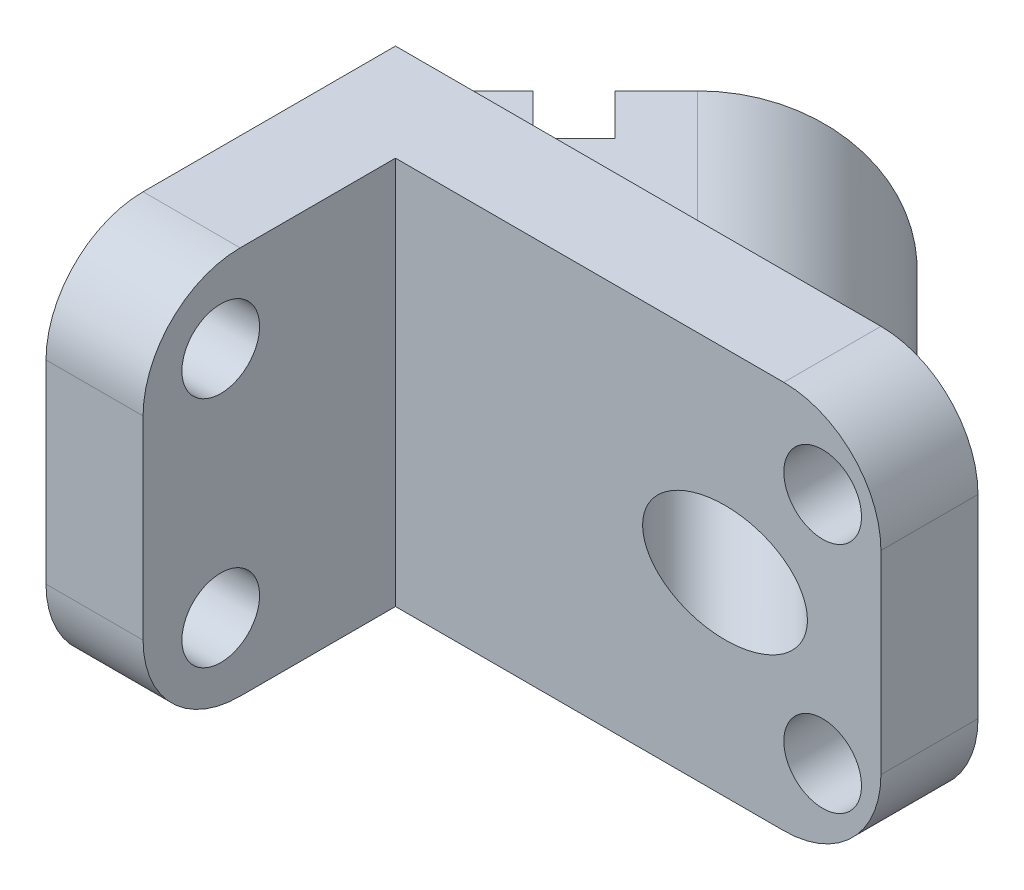
ISO-10303-21;
HEADER;
FILE_DESCRIPTION(('STEP AP214'),'2;1');
FILE_NAME('part.step','',(''),(''),'','','');
FILE_SCHEMA(('AUTOMOTIVE_DESIGN { 1 0 10303 214 1 1 1 1 }'));
ENDSEC;
DATA;
#1=APPLICATION_CONTEXT('core data for automotive mechanical design processes');
#2=APPLICATION_PROTOCOL_DEFINITION('international standard','automotive_design',2000,#1);
#3=PRODUCT_CONTEXT('',#1,'mechanical');
#4=PRODUCT('Part','Part','',(#3));
#5=PRODUCT_RELATED_PRODUCT_CATEGORY('part','',(#4));
#6=PRODUCT_DEFINITION_FORMATION('','',#4);
#7=PRODUCT_DEFINITION_CONTEXT('part definition',#1,'design');
#8=PRODUCT_DEFINITION('design','',#6,#7);
#9=PRODUCT_DEFINITION_SHAPE('','',#8);
#10=(LENGTH_UNIT() NAMED_UNIT(*) SI_UNIT(.MILLI.,.METRE.));
#11=(NAMED_UNIT(*) PLANE_ANGLE_UNIT() SI_UNIT($,.RADIAN.));
#12=(NAMED_UNIT(*) SI_UNIT($,.STERADIAN.) SOLID_ANGLE_UNIT());
#13=UNCERTAINTY_MEASURE_WITH_UNIT(LENGTH_MEASURE(1.E-05),#10,'distance_accuracy_value','');
#14=(GEOMETRIC_REPRESENTATION_CONTEXT(3) GLOBAL_UNCERTAINTY_ASSIGNED_CONTEXT((#13)) GLOBAL_UNIT_ASSIGNED_CONTEXT((#10,
#11,#12)) REPRESENTATION_CONTEXT('',''));
#15=CARTESIAN_POINT('',(0.,0.,0.));
#16=DIRECTION('',(0.,0.,1.));
#17=DIRECTION('',(1.,0.,0.));
#18=AXIS2_PLACEMENT_3D('',#15,#16,#17);
#19=CARTESIAN_POINT('',(-36.1091270347396,0.,-38.8908729652601));
#20=DIRECTION('',(0.707106781186544,0.,0.707106781186551));
#21=DIRECTION('',(0.707106781186551,0.,-0.707106781186544));
#22=AXIS2_PLACEMENT_3D('',#19,#20,#21);
#23=PLANE('',#22);
#24=DIRECTION('',(-0.707106781186551,0.,0.707106781186544));
#25=VECTOR('',#24,1.);
#26=CARTESIAN_POINT('',(-74.9999999999999,40.,-1.38777878078145E-13));
#27=LINE('',#26,#25);
#28=CARTESIAN_POINT('',(-57.3223304703362,40.,-17.6776695296636));
#29=VERTEX_POINT('',#28);
#30=CARTESIAN_POINT('',(-75.,40.,0.));
#31=VERTEX_POINT('',#30);
#32=EDGE_CURVE('E201',#29,#31,#27,.T.);
#33=ORIENTED_EDGE('',*,*,#32,.F.);
#34=DIRECTION('',(0.,1.,0.));
#35=VECTOR('',#34,1.);
#36=CARTESIAN_POINT('',(-57.3223304703362,-50.001,-17.6776695296636));
#37=LINE('',#36,#35);
#38=CARTESIAN_POINT('',(-57.3223304703362,-40.,-17.6776695296636));
#39=VERTEX_POINT('',#38);
#40=EDGE_CURVE('E200',#39,#29,#37,.T.);
#41=ORIENTED_EDGE('',*,*,#40,.F.);
#42=DIRECTION('',(0.707106781186551,0.,-0.707106781186544));
#43=VECTOR('',#42,1.);
#44=CARTESIAN_POINT('',(-74.9999999999999,-40.,-1.38777878078145E-13));
#45=LINE('',#44,#43);
#46=CARTESIAN_POINT('',(-74.9999999999999,-40.,-1.38777878078145E-13));
#47=VERTEX_POINT('',#46);
#48=EDGE_CURVE('E202',#47,#39,#45,.T.);
#49=ORIENTED_EDGE('',*,*,#48,.F.);
#50=DIRECTION('',(0.,-1.,0.));
#51=VECTOR('',#50,1.);
#52=CARTESIAN_POINT('',(-74.9999999999999,40.,-1.38777878078145E-13));
#53=LINE('',#52,#51);
#54=EDGE_CURVE('E207',#31,#47,#53,.T.);
#55=ORIENTED_EDGE('',*,*,#54,.F.);
#56=EDGE_LOOP('',(#33,#41,#49,#55));
#57=FACE_BOUND('',#56,.T.);
#58=ADVANCED_FACE('F39',(#57),#23,.F.);
#59=CARTESIAN_POINT('',(0.,0.,25.));
#60=DIRECTION('',(0.,0.,-1.));
#61=DIRECTION('',(-1.,0.,0.));
#62=AXIS2_PLACEMENT_3D('',#59,#60,#61);
#63=PLANE('',#62);
#64=CARTESIAN_POINT('',(60.,30.,25.));
#65=DIRECTION('',(0.,0.,-1.));
#66=DIRECTION('',(-1.,0.,0.));
#67=AXIS2_PLACEMENT_3D('',#64,#65,#66);
#68=CIRCLE('',#67,10.);
#69=CARTESIAN_POINT('',(50.,30.,25.));
#70=VERTEX_POINT('',#69);
#71=EDGE_CURVE('E597',#70,#70,#68,.F.);
#72=ORIENTED_EDGE('',*,*,#71,.F.);
#73=EDGE_LOOP('',(#72));
#74=FACE_BOUND('',#73,.T.);
#75=CARTESIAN_POINT('',(60.,-30.,25.));
#76=DIRECTION('',(0.,0.,-1.));
#77=DIRECTION('',(-1.,0.,0.));
#78=AXIS2_PLACEMENT_3D('',#75,#76,#77);
#79=CIRCLE('',#78,10.);
#80=CARTESIAN_POINT('',(50.,-30.,25.));
#81=VERTEX_POINT('',#80);
#82=EDGE_CURVE('E585',#81,#81,#79,.F.);
#83=ORIENTED_EDGE('',*,*,#82,.F.);
#84=EDGE_LOOP('',(#83));
#85=FACE_BOUND('',#84,.T.);
#86=CARTESIAN_POINT('',(34.852813742385,0.,25.));
#87=DIRECTION('',(0.,0.,-1.));
#88=DIRECTION('',(-1.,0.,0.));
#89=AXIS2_PLACEMENT_3D('',#86,#87,#88);
#90=ELLIPSE('',#89,21.2132034355963,15.);
#91=CARTESIAN_POINT('',(13.6396103067887,0.,25.));
#92=VERTEX_POINT('',#91);
#93=EDGE_CURVE('E182',#92,#92,#90,.F.);
#94=ORIENTED_EDGE('',*,*,#93,.F.);
#95=EDGE_LOOP('',(#94));
#96=FACE_BOUND('',#95,.T.);
#97=DIRECTION('',(0.,1.,0.));
#98=VECTOR('',#97,1.);
#99=CARTESIAN_POINT('',(75.,-50.,25.));
#100=LINE('',#99,#98);
#101=CARTESIAN_POINT('',(75.,-25.,25.));
#102=VERTEX_POINT('',#101);
#103=CARTESIAN_POINT('',(75.,25.,25.));
#104=VERTEX_POINT('',#103);
#105=EDGE_CURVE('E237',#102,#104,#100,.T.);
#106=ORIENTED_EDGE('',*,*,#105,.T.);
#107=CARTESIAN_POINT('',(50.,25.,25.));
#108=DIRECTION('',(0.,0.,-1.));
#109=DIRECTION('',(-1.,0.,0.));
#110=AXIS2_PLACEMENT_3D('',#107,#108,#109);
#111=CIRCLE('',#110,25.);
#112=CARTESIAN_POINT('',(50.,50.,25.));
#113=VERTEX_POINT('',#112);
#114=EDGE_CURVE('E11',#104,#113,#111,.F.);
#115=ORIENTED_EDGE('',*,*,#114,.T.);
#116=DIRECTION('',(-1.,0.,0.));
#117=VECTOR('',#116,1.);
#118=CARTESIAN_POINT('',(-75.,50.,25.));
#119=LINE('',#118,#117);
#120=CARTESIAN_POINT('',(-50.,50.,25.));
#121=VERTEX_POINT('',#120);
#122=EDGE_CURVE('E241',#113,#121,#119,.T.);
#123=ORIENTED_EDGE('',*,*,#122,.T.);
#124=DIRECTION('',(0.,1.,0.));
#125=VECTOR('',#124,1.);
#126=CARTESIAN_POINT('',(-50.,50.,25.));
#127=LINE('',#126,#125);
#128=CARTESIAN_POINT('',(-50.,-50.,25.));
#129=VERTEX_POINT('',#128);
#130=EDGE_CURVE('E206',#129,#121,#127,.T.);
#131=ORIENTED_EDGE('',*,*,#130,.F.);
#132=DIRECTION('',(1.,0.,0.));
#133=VECTOR('',#132,1.);
#134=CARTESIAN_POINT('',(-75.,-50.,25.));
#135=LINE('',#134,#133);
#136=CARTESIAN_POINT('',(50.,-50.,25.));
#137=VERTEX_POINT('',#136);
#138=EDGE_CURVE('E242',#129,#137,#135,.T.);
#139=ORIENTED_EDGE('',*,*,#138,.T.);
#140=CARTESIAN_POINT('',(50.,-25.,25.));
#141=DIRECTION('',(0.,0.,-1.));
#142=DIRECTION('',(-1.,0.,0.));
#143=AXIS2_PLACEMENT_3D('',#140,#141,#142);
#144=CIRCLE('',#143,25.);
#145=EDGE_CURVE('E290',#137,#102,#144,.F.);
#146=ORIENTED_EDGE('',*,*,#145,.T.);
#147=EDGE_LOOP('',(#106,#115,#123,#131,#139,#146));
#148=FACE_BOUND('',#147,.T.);
#149=ADVANCED_FACE('F337',(#74,#85,#96,#148),#63,.F.);
#150=CARTESIAN_POINT('',(75.,-50.,25.));
#151=DIRECTION('',(-1.,0.,0.));
#152=DIRECTION('',(0.,0.,1.));
#153=AXIS2_PLACEMENT_3D('',#150,#151,#152);
#154=PLANE('',#153);
#155=DIRECTION('',(0.,1.,0.));
#156=VECTOR('',#155,1.);
#157=CARTESIAN_POINT('',(75.,-50.,0.));
#158=LINE('',#157,#156);
#159=CARTESIAN_POINT('',(75.,-25.,0.));
#160=VERTEX_POINT('',#159);
#161=CARTESIAN_POINT('',(75.,25.,0.));
#162=VERTEX_POINT('',#161);
#163=EDGE_CURVE('E238',#160,#162,#158,.T.);
#164=ORIENTED_EDGE('',*,*,#163,.T.);
#165=DIRECTION('',(0.,0.,-1.));
#166=VECTOR('',#165,1.);
#167=CARTESIAN_POINT('',(75.,25.,25.));
#168=LINE('',#167,#166);
#169=EDGE_CURVE('E50',#162,#104,#168,.F.);
#170=ORIENTED_EDGE('',*,*,#169,.T.);
#171=ORIENTED_EDGE('',*,*,#105,.F.);
#172=DIRECTION('',(0.,0.,-1.));
#173=VECTOR('',#172,1.);
#174=CARTESIAN_POINT('',(75.,-25.,25.));
#175=LINE('',#174,#173);
#176=EDGE_CURVE('E277',#102,#160,#175,.T.);
#177=ORIENTED_EDGE('',*,*,#176,.T.);
#178=EDGE_LOOP('',(#164,#170,#171,#177));
#179=FACE_BOUND('',#178,.T.);
#180=ADVANCED_FACE('F345',(#179),#154,.F.);
#181=CARTESIAN_POINT('',(-75.,50.,25.));
#182=DIRECTION('',(0.,-1.,0.));
#183=DIRECTION('',(0.,0.,-1.));
#184=AXIS2_PLACEMENT_3D('',#181,#182,#183);
#185=PLANE('',#184);
#186=ORIENTED_EDGE('',*,*,#122,.F.);
#187=DIRECTION('',(0.,0.,-1.));
#188=VECTOR('',#187,1.);
#189=CARTESIAN_POINT('',(50.,50.,25.));
#190=LINE('',#189,#188);
#191=CARTESIAN_POINT('',(50.,50.,0.));
#192=VERTEX_POINT('',#191);
#193=EDGE_CURVE('E287',#113,#192,#190,.T.);
#194=ORIENTED_EDGE('',*,*,#193,.T.);
#195=DIRECTION('',(-1.,0.,0.));
#196=VECTOR('',#195,1.);
#197=CARTESIAN_POINT('',(-75.,50.,0.));
#198=LINE('',#197,#196);
#199=CARTESIAN_POINT('',(-75.,50.,0.));
#200=VERTEX_POINT('',#199);
#201=EDGE_CURVE('E248',#192,#200,#198,.T.);
#202=ORIENTED_EDGE('',*,*,#201,.T.);
#203=DIRECTION('',(0.,0.,-1.));
#204=VECTOR('',#203,1.);
#205=CARTESIAN_POINT('',(-75.,50.,25.));
#206=LINE('',#205,#204);
#207=CARTESIAN_POINT('',(-75.,50.,65.));
#208=VERTEX_POINT('',#207);
#209=EDGE_CURVE('E260',#208,#200,#206,.T.);
#210=ORIENTED_EDGE('',*,*,#209,.F.);
#211=DIRECTION('',(-1.,0.,0.));
#212=VECTOR('',#211,1.);
#213=CARTESIAN_POINT('',(-50.,50.,65.));
#214=LINE('',#213,#212);
#215=CARTESIAN_POINT('',(-50.,50.,65.));
#216=VERTEX_POINT('',#215);
#217=EDGE_CURVE('E268',#208,#216,#214,.F.);
#218=ORIENTED_EDGE('',*,*,#217,.T.);
#219=DIRECTION('',(0.,0.,-1.));
#220=VECTOR('',#219,1.);
#221=CARTESIAN_POINT('',(-50.,50.,90.));
#222=LINE('',#221,#220);
#223=EDGE_CURVE('E233',#216,#121,#222,.T.);
#224=ORIENTED_EDGE('',*,*,#223,.T.);
#225=EDGE_LOOP('',(#186,#194,#202,#210,#218,#224));
#226=FACE_BOUND('',#225,.T.);
#227=ADVANCED_FACE('F294',(#226),#185,.F.);
#228=CARTESIAN_POINT('',(-75.,-50.,25.));
#229=DIRECTION('',(1.,0.,0.));
#230=DIRECTION('',(0.,0.,-1.));
#231=AXIS2_PLACEMENT_3D('',#228,#229,#230);
#232=PLANE('',#231);
#233=CARTESIAN_POINT('',(-75.,30.,70.));
#234=DIRECTION('',(-1.,0.,0.));
#235=DIRECTION('',(0.,0.,1.));
#236=AXIS2_PLACEMENT_3D('',#233,#234,#235);
#237=CIRCLE('',#236,9.99999999999999);
#238=CARTESIAN_POINT('',(-75.,30.,80.));
#239=VERTEX_POINT('',#238);
#240=EDGE_CURVE('E577',#239,#239,#237,.T.);
#241=ORIENTED_EDGE('',*,*,#240,.F.);
#242=EDGE_LOOP('',(#241));
#243=FACE_BOUND('',#242,.T.);
#244=CARTESIAN_POINT('',(-75.,-30.,70.));
#245=DIRECTION('',(-1.,0.,0.));
#246=DIRECTION('',(0.,0.,1.));
#247=AXIS2_PLACEMENT_3D('',#244,#245,#246);
#248=CIRCLE('',#247,9.99999999999999);
#249=CARTESIAN_POINT('',(-75.,-30.,80.));
#250=VERTEX_POINT('',#249);
#251=EDGE_CURVE('E587',#250,#250,#248,.T.);
#252=ORIENTED_EDGE('',*,*,#251,.F.);
#253=EDGE_LOOP('',(#252));
#254=FACE_BOUND('',#253,.T.);
#255=DIRECTION('',(0.,0.,-1.));
#256=VECTOR('',#255,1.);
#257=CARTESIAN_POINT('',(-75.,-50.,25.));
#258=LINE('',#257,#256);
#259=CARTESIAN_POINT('',(-75.,-50.,65.));
#260=VERTEX_POINT('',#259);
#261=CARTESIAN_POINT('',(-75.,-50.,0.));
#262=VERTEX_POINT('',#261);
#263=EDGE_CURVE('E250',#260,#262,#258,.T.);
#264=ORIENTED_EDGE('',*,*,#263,.F.);
#265=CARTESIAN_POINT('',(-75.,-25.,65.));
#266=DIRECTION('',(1.,0.,0.));
#267=DIRECTION('',(0.,0.,-1.));
#268=AXIS2_PLACEMENT_3D('',#265,#266,#267);
#269=CIRCLE('',#268,25.);
#270=CARTESIAN_POINT('',(-75.,-25.,90.));
#271=VERTEX_POINT('',#270);
#272=EDGE_CURVE('E280',#260,#271,#269,.F.);
#273=ORIENTED_EDGE('',*,*,#272,.T.);
#274=DIRECTION('',(0.,-1.,0.));
#275=VECTOR('',#274,1.);
#276=CARTESIAN_POINT('',(-75.,50.,90.));
#277=LINE('',#276,#275);
#278=CARTESIAN_POINT('',(-75.,25.,90.));
#279=VERTEX_POINT('',#278);
#280=EDGE_CURVE('E228',#279,#271,#277,.T.);
#281=ORIENTED_EDGE('',*,*,#280,.F.);
#282=CARTESIAN_POINT('',(-75.,25.,65.));
#283=DIRECTION('',(1.,0.,0.));
#284=DIRECTION('',(0.,0.,-1.));
#285=AXIS2_PLACEMENT_3D('',#282,#283,#284);
#286=CIRCLE('',#285,25.);
#287=EDGE_CURVE('E263',#279,#208,#286,.F.);
#288=ORIENTED_EDGE('',*,*,#287,.T.);
#289=ORIENTED_EDGE('',*,*,#209,.T.);
#290=DIRECTION('',(0.,-1.,0.));
#291=VECTOR('',#290,1.);
#292=CARTESIAN_POINT('',(-75.,-50.,0.));
#293=LINE('',#292,#291);
#294=EDGE_CURVE('E255',#200,#31,#293,.T.);
#295=ORIENTED_EDGE('',*,*,#294,.T.);
#296=ORIENTED_EDGE('',*,*,#54,.T.);
#297=EDGE_CURVE('E252',#47,#262,#293,.T.);
#298=ORIENTED_EDGE('',*,*,#297,.T.);
#299=EDGE_LOOP('',(#264,#273,#281,#288,#289,#295,#296,#298));
#300=FACE_BOUND('',#299,.T.);
#301=ADVANCED_FACE('F304',(#243,#254,#300),#232,.F.);
#302=CARTESIAN_POINT('',(-75.,-50.,25.));
#303=DIRECTION('',(0.,1.,0.));
#304=DIRECTION('',(0.,0.,1.));
#305=AXIS2_PLACEMENT_3D('',#302,#303,#304);
#306=PLANE('',#305);
#307=DIRECTION('',(1.,0.,0.));
#308=VECTOR('',#307,1.);
#309=CARTESIAN_POINT('',(-75.,-50.,0.));
#310=LINE('',#309,#308);
#311=CARTESIAN_POINT('',(50.,-50.,0.));
#312=VERTEX_POINT('',#311);
#313=EDGE_CURVE('E245',#262,#312,#310,.T.);
#314=ORIENTED_EDGE('',*,*,#313,.T.);
#315=DIRECTION('',(0.,0.,-1.));
#316=VECTOR('',#315,1.);
#317=CARTESIAN_POINT('',(50.,-50.,25.));
#318=LINE('',#317,#316);
#319=EDGE_CURVE('E284',#312,#137,#318,.F.);
#320=ORIENTED_EDGE('',*,*,#319,.T.);
#321=ORIENTED_EDGE('',*,*,#138,.F.);
#322=DIRECTION('',(0.,0.,-1.));
#323=VECTOR('',#322,1.);
#324=CARTESIAN_POINT('',(-50.,-50.,90.));
#325=LINE('',#324,#323);
#326=CARTESIAN_POINT('',(-50.,-50.,65.));
#327=VERTEX_POINT('',#326);
#328=EDGE_CURVE('E236',#327,#129,#325,.T.);
#329=ORIENTED_EDGE('',*,*,#328,.F.);
#330=DIRECTION('',(1.,0.,0.));
#331=VECTOR('',#330,1.);
#332=CARTESIAN_POINT('',(-75.,-50.,65.));
#333=LINE('',#332,#331);
#334=EDGE_CURVE('E279',#327,#260,#333,.F.);
#335=ORIENTED_EDGE('',*,*,#334,.T.);
#336=ORIENTED_EDGE('',*,*,#263,.T.);
#337=EDGE_LOOP('',(#314,#320,#321,#329,#335,#336));
#338=FACE_BOUND('',#337,.T.);
#339=ADVANCED_FACE('F371',(#338),#306,.F.);
#340=CARTESIAN_POINT('',(0.,0.,0.));
#341=DIRECTION('',(0.,0.,-1.));
#342=DIRECTION('',(-1.,0.,0.));
#343=AXIS2_PLACEMENT_3D('',#340,#341,#342);
#344=PLANE('',#343);
#345=CARTESIAN_POINT('',(60.,30.,0.));
#346=DIRECTION('',(0.,0.,-1.));
#347=DIRECTION('',(-1.,0.,0.));
#348=AXIS2_PLACEMENT_3D('',#345,#346,#347);
#349=CIRCLE('',#348,10.);
#350=CARTESIAN_POINT('',(50.,30.,0.));
#351=VERTEX_POINT('',#350);
#352=EDGE_CURVE('E591',#351,#351,#349,.T.);
#353=ORIENTED_EDGE('',*,*,#352,.F.);
#354=EDGE_LOOP('',(#353));
#355=FACE_BOUND('',#354,.T.);
#356=CARTESIAN_POINT('',(60.,-30.,0.));
#357=DIRECTION('',(0.,0.,-1.));
#358=DIRECTION('',(-1.,0.,0.));
#359=AXIS2_PLACEMENT_3D('',#356,#357,#358);
#360=CIRCLE('',#359,10.);
#361=CARTESIAN_POINT('',(50.,-30.,0.));
#362=VERTEX_POINT('',#361);
#363=EDGE_CURVE('E578',#362,#362,#360,.T.);
#364=ORIENTED_EDGE('',*,*,#363,.F.);
#365=EDGE_LOOP('',(#364));
#366=FACE_BOUND('',#365,.T.);
#367=ORIENTED_EDGE('',*,*,#201,.F.);
#368=CARTESIAN_POINT('',(50.,25.,0.));
#369=DIRECTION('',(0.,0.,-1.));
#370=DIRECTION('',(-1.,0.,0.));
#371=AXIS2_PLACEMENT_3D('',#368,#369,#370);
#372=CIRCLE('',#371,25.);
#373=EDGE_CURVE('E64',#192,#162,#372,.T.);
#374=ORIENTED_EDGE('',*,*,#373,.T.);
#375=ORIENTED_EDGE('',*,*,#163,.F.);
#376=CARTESIAN_POINT('',(50.,-25.,0.));
#377=DIRECTION('',(0.,0.,-1.));
#378=DIRECTION('',(-1.,0.,0.));
#379=AXIS2_PLACEMENT_3D('',#376,#377,#378);
#380=CIRCLE('',#379,25.);
#381=EDGE_CURVE('E282',#160,#312,#380,.T.);
#382=ORIENTED_EDGE('',*,*,#381,.T.);
#383=ORIENTED_EDGE('',*,*,#313,.F.);
#384=ORIENTED_EDGE('',*,*,#297,.F.);
#385=DIRECTION('',(-1.,0.,0.));
#386=VECTOR('',#385,1.);
#387=CARTESIAN_POINT('',(12.5014142135617,-40.,0.));
#388=LINE('',#387,#386);
#389=CARTESIAN_POINT('',(2.78174593052008,-40.,0.));
#390=VERTEX_POINT('',#389);
#391=EDGE_CURVE('E209',#390,#47,#388,.T.);
#392=ORIENTED_EDGE('',*,*,#391,.F.);
#393=CARTESIAN_POINT('',(2.78174593052009,0.,0.));
#394=DIRECTION('',(0.,0.,-1.));
#395=DIRECTION('',(-1.,0.,0.));
#396=AXIS2_PLACEMENT_3D('',#393,#394,#395);
#397=ELLIPSE('',#396,56.5685424949235,40.);
#398=CARTESIAN_POINT('',(2.78174593052009,40.,0.));
#399=VERTEX_POINT('',#398);
#400=EDGE_CURVE('E223',#399,#390,#397,.T.);
#401=ORIENTED_EDGE('',*,*,#400,.F.);
#402=DIRECTION('',(1.,0.,0.));
#403=VECTOR('',#402,1.);
#404=CARTESIAN_POINT('',(12.5014142135617,40.,0.));
#405=LINE('',#404,#403);
#406=EDGE_CURVE('E220',#31,#399,#405,.T.);
#407=ORIENTED_EDGE('',*,*,#406,.F.);
#408=ORIENTED_EDGE('',*,*,#294,.F.);
#409=EDGE_LOOP('',(#367,#374,#375,#382,#383,#384,#392,#401,#407,#408));
#410=FACE_BOUND('',#409,.T.);
#411=ADVANCED_FACE('F297',(#355,#366,#410),#344,.T.);
#412=CARTESIAN_POINT('',(-50.,50.,90.));
#413=DIRECTION('',(-1.,0.,0.));
#414=DIRECTION('',(0.,-1.,0.));
#415=AXIS2_PLACEMENT_3D('',#412,#413,#414);
#416=PLANE('',#415);
#417=CARTESIAN_POINT('',(-50.,30.,70.));
#418=DIRECTION('',(-1.,0.,0.));
#419=DIRECTION('',(0.,-1.,0.));
#420=AXIS2_PLACEMENT_3D('',#417,#418,#419);
#421=CIRCLE('',#420,9.99999999999999);
#422=CARTESIAN_POINT('',(-50.,20.,70.));
#423=VERTEX_POINT('',#422);
#424=EDGE_CURVE('E576',#423,#423,#421,.F.);
#425=ORIENTED_EDGE('',*,*,#424,.F.);
#426=EDGE_LOOP('',(#425));
#427=FACE_BOUND('',#426,.T.);
#428=CARTESIAN_POINT('',(-50.,-30.,70.));
#429=DIRECTION('',(-1.,0.,0.));
#430=DIRECTION('',(0.,-1.,0.));
#431=AXIS2_PLACEMENT_3D('',#428,#429,#430);
#432=CIRCLE('',#431,9.99999999999999);
#433=CARTESIAN_POINT('',(-50.,-40.,70.));
#434=VERTEX_POINT('',#433);
#435=EDGE_CURVE('E582',#434,#434,#432,.F.);
#436=ORIENTED_EDGE('',*,*,#435,.F.);
#437=EDGE_LOOP('',(#436));
#438=FACE_BOUND('',#437,.T.);
#439=DIRECTION('',(0.,1.,0.));
#440=VECTOR('',#439,1.);
#441=CARTESIAN_POINT('',(-50.,50.,90.));
#442=LINE('',#441,#440);
#443=CARTESIAN_POINT('',(-50.,-25.,90.));
#444=VERTEX_POINT('',#443);
#445=CARTESIAN_POINT('',(-50.,25.,90.));
#446=VERTEX_POINT('',#445);
#447=EDGE_CURVE('E230',#444,#446,#442,.T.);
#448=ORIENTED_EDGE('',*,*,#447,.F.);
#449=CARTESIAN_POINT('',(-50.,-25.,65.));
#450=DIRECTION('',(-1.,0.,0.));
#451=DIRECTION('',(0.,-1.,0.));
#452=AXIS2_PLACEMENT_3D('',#449,#450,#451);
#453=CIRCLE('',#452,25.);
#454=EDGE_CURVE('E274',#444,#327,#453,.F.);
#455=ORIENTED_EDGE('',*,*,#454,.T.);
#456=ORIENTED_EDGE('',*,*,#328,.T.);
#457=ORIENTED_EDGE('',*,*,#130,.T.);
#458=ORIENTED_EDGE('',*,*,#223,.F.);
#459=CARTESIAN_POINT('',(-50.,25.,65.));
#460=DIRECTION('',(-1.,0.,0.));
#461=DIRECTION('',(0.,-1.,0.));
#462=AXIS2_PLACEMENT_3D('',#459,#460,#461);
#463=CIRCLE('',#462,25.);
#464=EDGE_CURVE('E266',#216,#446,#463,.F.);
#465=ORIENTED_EDGE('',*,*,#464,.T.);
#466=EDGE_LOOP('',(#448,#455,#456,#457,#458,#465));
#467=FACE_BOUND('',#466,.T.);
#468=ADVANCED_FACE('F357',(#427,#438,#467),#416,.F.);
#469=CARTESIAN_POINT('',(0.,0.,90.));
#470=DIRECTION('',(0.,0.,1.));
#471=DIRECTION('',(1.,0.,0.));
#472=AXIS2_PLACEMENT_3D('',#469,#470,#471);
#473=PLANE('',#472);
#474=ORIENTED_EDGE('',*,*,#280,.T.);
#475=DIRECTION('',(1.,0.,0.));
#476=VECTOR('',#475,1.);
#477=CARTESIAN_POINT('',(-50.,-25.,90.));
#478=LINE('',#477,#476);
#479=EDGE_CURVE('E272',#271,#444,#478,.T.);
#480=ORIENTED_EDGE('',*,*,#479,.T.);
#481=ORIENTED_EDGE('',*,*,#447,.T.);
#482=DIRECTION('',(-1.,0.,0.));
#483=VECTOR('',#482,1.);
#484=CARTESIAN_POINT('',(-75.,25.,90.));
#485=LINE('',#484,#483);
#486=EDGE_CURVE('E261',#446,#279,#485,.T.);
#487=ORIENTED_EDGE('',*,*,#486,.T.);
#488=EDGE_LOOP('',(#474,#480,#481,#487));
#489=FACE_BOUND('',#488,.T.);
#490=ADVANCED_FACE('F348',(#489),#473,.T.);
#491=CARTESIAN_POINT('',(12.5014142135617,-40.,87.5014142135624));
#492=DIRECTION('',(0.,1.,0.));
#493=DIRECTION('',(0.,0.,1.));
#494=AXIS2_PLACEMENT_3D('',#491,#492,#493);
#495=PLANE('',#494);
#496=ORIENTED_EDGE('',*,*,#48,.T.);
#497=DIRECTION('',(-0.707106781186527,0.,-0.707106781186568));
#498=VECTOR('',#497,1.);
#499=CARTESIAN_POINT('',(-57.3223304703362,-40.,-17.6776695296636));
#500=LINE('',#499,#498);
#501=CARTESIAN_POINT('',(-46.7157287525383,-40.,-7.07106781186509));
#502=VERTEX_POINT('',#501);
#503=EDGE_CURVE('E185',#502,#39,#500,.T.);
#504=ORIENTED_EDGE('',*,*,#503,.F.);
#505=DIRECTION('',(-0.707106781186527,0.,0.707106781186568));
#506=VECTOR('',#505,1.);
#507=CARTESIAN_POINT('',(-46.7157287525383,-40.,-7.07106781186509));
#508=LINE('',#507,#506);
#509=CARTESIAN_POINT('',(-36.1091270347404,-40.,-17.6776695296636));
#510=VERTEX_POINT('',#509);
#511=EDGE_CURVE('E162',#510,#502,#508,.T.);
#512=ORIENTED_EDGE('',*,*,#511,.F.);
#513=DIRECTION('',(0.707106781186551,0.,0.707106781186544));
#514=VECTOR('',#513,1.);
#515=CARTESIAN_POINT('',(-36.1091270347404,-40.,-17.6776695296636));
#516=LINE('',#515,#514);
#517=CARTESIAN_POINT('',(-46.7157287525383,-40.,-28.2842712474614));
#518=VERTEX_POINT('',#517);
#519=EDGE_CURVE('E175',#518,#510,#516,.T.);
#520=ORIENTED_EDGE('',*,*,#519,.F.);
#521=CARTESIAN_POINT('',(-36.1091270347396,-40.,-38.89087296526));
#522=VERTEX_POINT('',#521);
#523=EDGE_CURVE('E180',#518,#522,#45,.T.);
#524=ORIENTED_EDGE('',*,*,#523,.T.);
#525=DIRECTION('',(-0.707106781186544,0.,-0.707106781186551));
#526=VECTOR('',#525,1.);
#527=CARTESIAN_POINT('',(51.392287178822,-40.,48.6105412483025));
#528=LINE('',#527,#526);
#529=EDGE_CURVE('E213',#390,#522,#528,.T.);
#530=ORIENTED_EDGE('',*,*,#529,.F.);
#531=ORIENTED_EDGE('',*,*,#391,.T.);
#532=EDGE_LOOP('',(#496,#504,#512,#520,#524,#530,#531));
#533=FACE_BOUND('',#532,.T.);
#534=ADVANCED_FACE('F181',(#533),#495,.F.);
#535=CARTESIAN_POINT('',(51.392287178822,0.,48.6105412483025));
#536=DIRECTION('',(-0.707106781186544,0.,-0.707106781186551));
#537=DIRECTION('',(-0.707106781186551,0.,0.707106781186544));
#538=AXIS2_PLACEMENT_3D('',#535,#536,#537);
#539=CYLINDRICAL_SURFACE('',#538,40.);
#540=DIRECTION('',(-0.707106781186544,0.,-0.707106781186551));
#541=VECTOR('',#540,1.);
#542=CARTESIAN_POINT('',(51.392287178822,40.,48.6105412483025));
#543=LINE('',#542,#541);
#544=CARTESIAN_POINT('',(-36.1091270347396,40.,-38.8908729652601));
#545=VERTEX_POINT('',#544);
#546=EDGE_CURVE('E215',#399,#545,#543,.T.);
#547=ORIENTED_EDGE('',*,*,#546,.F.);
#548=ORIENTED_EDGE('',*,*,#400,.T.);
#549=ORIENTED_EDGE('',*,*,#529,.T.);
#550=CARTESIAN_POINT('',(-36.1091270347396,0.,-38.8908729652601));
#551=DIRECTION('',(0.707106781186544,0.,0.707106781186551));
#552=DIRECTION('',(0.707106781186551,0.,-0.707106781186544));
#553=AXIS2_PLACEMENT_3D('',#550,#551,#552);
#554=CIRCLE('',#553,40.);
#555=EDGE_CURVE('E199',#522,#545,#554,.T.);
#556=ORIENTED_EDGE('',*,*,#555,.T.);
#557=EDGE_LOOP('',(#547,#548,#549,#556));
#558=FACE_BOUND('',#557,.T.);
#559=ADVANCED_FACE('F317',(#558),#539,.T.);
#560=CARTESIAN_POINT('',(12.5014142135617,40.,87.5014142135624));
#561=DIRECTION('',(0.,-1.,0.));
#562=DIRECTION('',(1.,0.,0.));
#563=AXIS2_PLACEMENT_3D('',#560,#561,#562);
#564=PLANE('',#563);
#565=DIRECTION('',(0.707106781186527,0.,-0.707106781186568));
#566=VECTOR('',#565,1.);
#567=CARTESIAN_POINT('',(-46.7157287525383,40.,-7.0710678118651));
#568=LINE('',#567,#566);
#569=CARTESIAN_POINT('',(-46.7157287525383,40.,-7.0710678118651));
#570=VERTEX_POINT('',#569);
#571=CARTESIAN_POINT('',(-36.1091270347404,40.,-17.6776695296636));
#572=VERTEX_POINT('',#571);
#573=EDGE_CURVE('E164',#570,#572,#568,.T.);
#574=ORIENTED_EDGE('',*,*,#573,.F.);
#575=DIRECTION('',(0.707106781186527,0.,0.707106781186568));
#576=VECTOR('',#575,1.);
#577=CARTESIAN_POINT('',(-57.3223304703362,40.,-17.6776695296636));
#578=LINE('',#577,#576);
#579=EDGE_CURVE('E169',#29,#570,#578,.T.);
#580=ORIENTED_EDGE('',*,*,#579,.F.);
#581=ORIENTED_EDGE('',*,*,#32,.T.);
#582=ORIENTED_EDGE('',*,*,#406,.T.);
#583=ORIENTED_EDGE('',*,*,#546,.T.);
#584=CARTESIAN_POINT('',(-46.7157287525383,40.,-28.2842712474614));
#585=VERTEX_POINT('',#584);
#586=EDGE_CURVE('E208',#545,#585,#27,.T.);
#587=ORIENTED_EDGE('',*,*,#586,.T.);
#588=DIRECTION('',(-0.707106781186551,0.,-0.707106781186544));
#589=VECTOR('',#588,1.);
#590=CARTESIAN_POINT('',(-36.1091270347404,40.,-17.6776695296636));
#591=LINE('',#590,#589);
#592=EDGE_CURVE('E191',#572,#585,#591,.T.);
#593=ORIENTED_EDGE('',*,*,#592,.F.);
#594=EDGE_LOOP('',(#574,#580,#581,#582,#583,#587,#593));
#595=FACE_BOUND('',#594,.T.);
#596=ADVANCED_FACE('F318',(#595),#564,.F.);
#597=CARTESIAN_POINT('',(-32.5735931288069,0.,-42.4264068711927));
#598=DIRECTION('',(-0.707106781186544,0.,-0.707106781186551));
#599=DIRECTION('',(-0.707106781186551,0.,0.707106781186544));
#600=AXIS2_PLACEMENT_3D('',#597,#598,#599);
#601=CIRCLE('',#600,15.);
#602=CARTESIAN_POINT('',(-43.1801948466052,0.,-31.8198051533945));
#603=VERTEX_POINT('',#602);
#604=EDGE_CURVE('E190',#603,#603,#601,.T.);
#605=ORIENTED_EDGE('',*,*,#604,.F.);
#606=EDGE_LOOP('',(#605));
#607=FACE_BOUND('',#606,.T.);
#608=ORIENTED_EDGE('',*,*,#523,.F.);
#609=DIRECTION('',(0.,1.,0.));
#610=VECTOR('',#609,1.);
#611=CARTESIAN_POINT('',(-46.7157287525383,-50.001,-28.2842712474614));
#612=LINE('',#611,#610);
#613=EDGE_CURVE('E166',#518,#585,#612,.T.);
#614=ORIENTED_EDGE('',*,*,#613,.T.);
#615=ORIENTED_EDGE('',*,*,#586,.F.);
#616=ORIENTED_EDGE('',*,*,#555,.F.);
#617=EDGE_LOOP('',(#608,#614,#615,#616));
#618=FACE_BOUND('',#617,.T.);
#619=ADVANCED_FACE('F335',(#607,#618),#23,.F.);
#620=CARTESIAN_POINT('',(-46.7157287525383,-50.001,-7.07106781186509));
#621=DIRECTION('',(0.707106781186568,0.,0.707106781186528));
#622=DIRECTION('',(0.707106781186527,0.,-0.707106781186568));
#623=AXIS2_PLACEMENT_3D('',#620,#621,#622);
#624=PLANE('',#623);
#625=ORIENTED_EDGE('',*,*,#511,.T.);
#626=DIRECTION('',(0.,1.,0.));
#627=VECTOR('',#626,1.);
#628=CARTESIAN_POINT('',(-46.7157287525383,-50.001,-7.07106781186509));
#629=LINE('',#628,#627);
#630=EDGE_CURVE('E178',#502,#570,#629,.T.);
#631=ORIENTED_EDGE('',*,*,#630,.T.);
#632=ORIENTED_EDGE('',*,*,#573,.T.);
#633=DIRECTION('',(0.,1.,0.));
#634=VECTOR('',#633,1.);
#635=CARTESIAN_POINT('',(-36.1091270347404,-50.001,-17.6776695296636));
#636=LINE('',#635,#634);
#637=EDGE_CURVE('E156',#510,#572,#636,.T.);
#638=ORIENTED_EDGE('',*,*,#637,.F.);
#639=EDGE_LOOP('',(#625,#631,#632,#638));
#640=FACE_BOUND('',#639,.T.);
#641=ADVANCED_FACE('F159',(#640),#624,.F.);
#642=CARTESIAN_POINT('',(-57.3223304703362,-50.001,-17.6776695296636));
#643=DIRECTION('',(-0.707106781186568,0.,0.707106781186528));
#644=DIRECTION('',(0.707106781186527,0.,0.707106781186568));
#645=AXIS2_PLACEMENT_3D('',#642,#643,#644);
#646=PLANE('',#645);
#647=ORIENTED_EDGE('',*,*,#503,.T.);
#648=ORIENTED_EDGE('',*,*,#40,.T.);
#649=ORIENTED_EDGE('',*,*,#579,.T.);
#650=ORIENTED_EDGE('',*,*,#630,.F.);
#651=EDGE_LOOP('',(#647,#648,#649,#650));
#652=FACE_BOUND('',#651,.T.);
#653=ADVANCED_FACE('F325',(#652),#646,.F.);
#654=CARTESIAN_POINT('',(-36.1091270347404,-50.001,-17.6776695296636));
#655=DIRECTION('',(0.707106781186544,0.,-0.707106781186551));
#656=DIRECTION('',(-0.707106781186551,0.,-0.707106781186544));
#657=AXIS2_PLACEMENT_3D('',#654,#655,#656);
#658=PLANE('',#657);
#659=ORIENTED_EDGE('',*,*,#519,.T.);
#660=ORIENTED_EDGE('',*,*,#637,.T.);
#661=ORIENTED_EDGE('',*,*,#592,.T.);
#662=ORIENTED_EDGE('',*,*,#613,.F.);
#663=EDGE_LOOP('',(#659,#660,#661,#662));
#664=FACE_BOUND('',#663,.T.);
#665=ADVANCED_FACE('F173',(#664),#658,.F.);
#666=CARTESIAN_POINT('',(87.4274068711923,0.,77.5745931288078));
#667=DIRECTION('',(-0.707106781186544,0.,-0.707106781186551));
#668=DIRECTION('',(-0.707106781186551,0.,0.707106781186544));
#669=AXIS2_PLACEMENT_3D('',#666,#667,#668);
#670=CYLINDRICAL_SURFACE('',#669,15.);
#671=ORIENTED_EDGE('',*,*,#604,.T.);
#672=EDGE_LOOP('',(#671));
#673=FACE_BOUND('',#672,.T.);
#674=ORIENTED_EDGE('',*,*,#93,.T.);
#675=EDGE_LOOP('',(#674));
#676=FACE_BOUND('',#675,.T.);
#677=ADVANCED_FACE('F329',(#673,#676),#670,.F.);
#678=CARTESIAN_POINT('',(60.,-30.,90.001));
#679=DIRECTION('',(0.,0.,-1.));
#680=DIRECTION('',(-1.,0.,0.));
#681=AXIS2_PLACEMENT_3D('',#678,#679,#680);
#682=CYLINDRICAL_SURFACE('',#681,10.);
#683=CARTESIAN_POINT('',(50.,-30.,0.));
#684=CARTESIAN_POINT('',(50.,-30.,0.260416666666679));
#685=CARTESIAN_POINT('',(50.,-30.,0.520833333333345));
#686=CARTESIAN_POINT('',(50.,-30.,1.04166666666668));
#687=CARTESIAN_POINT('',(50.,-30.,1.30208333333334));
#688=CARTESIAN_POINT('',(50.,-30.,1.82291666666668));
#689=CARTESIAN_POINT('',(50.,-30.,2.08333333333335));
#690=CARTESIAN_POINT('',(50.,-30.,2.60416666666669));
#691=CARTESIAN_POINT('',(50.,-30.,2.86458333333335));
#692=CARTESIAN_POINT('',(50.,-30.,3.38541666666668));
#693=CARTESIAN_POINT('',(50.,-30.,3.64583333333335));
#694=CARTESIAN_POINT('',(50.,-30.,4.16666666666668));
#695=CARTESIAN_POINT('',(50.,-30.,4.42708333333335));
#696=CARTESIAN_POINT('',(50.,-30.,4.94791666666668));
#697=CARTESIAN_POINT('',(50.,-30.,5.20833333333334));
#698=CARTESIAN_POINT('',(50.,-30.,5.72916666666668));
#699=CARTESIAN_POINT('',(50.,-30.,5.98958333333335));
#700=CARTESIAN_POINT('',(50.,-30.,6.51041666666669));
#701=CARTESIAN_POINT('',(50.,-30.,6.77083333333335));
#702=CARTESIAN_POINT('',(50.,-30.,7.29166666666668));
#703=CARTESIAN_POINT('',(50.,-30.,7.55208333333335));
#704=CARTESIAN_POINT('',(50.,-30.,8.07291666666668));
#705=CARTESIAN_POINT('',(50.,-30.,8.33333333333334));
#706=CARTESIAN_POINT('',(50.,-30.,8.85416666666668));
#707=CARTESIAN_POINT('',(50.,-30.,9.11458333333334));
#708=CARTESIAN_POINT('',(50.,-30.,9.63541666666668));
#709=CARTESIAN_POINT('',(50.,-30.,9.89583333333335));
#710=CARTESIAN_POINT('',(50.,-30.,10.4166666666667));
#711=CARTESIAN_POINT('',(50.,-30.,10.6770833333334));
#712=CARTESIAN_POINT('',(50.,-30.,11.1979166666667));
#713=CARTESIAN_POINT('',(50.,-30.,11.4583333333333));
#714=CARTESIAN_POINT('',(50.,-30.,11.9791666666667));
#715=CARTESIAN_POINT('',(50.,-30.,12.2395833333333));
#716=CARTESIAN_POINT('',(50.,-30.,12.7604166666667));
#717=CARTESIAN_POINT('',(50.,-30.,13.0208333333333));
#718=CARTESIAN_POINT('',(50.,-30.,13.5416666666667));
#719=CARTESIAN_POINT('',(50.,-30.,13.8020833333333));
#720=CARTESIAN_POINT('',(50.,-30.,14.3229166666667));
#721=CARTESIAN_POINT('',(50.,-30.,14.5833333333333));
#722=CARTESIAN_POINT('',(50.,-30.,15.1041666666667));
#723=CARTESIAN_POINT('',(50.,-30.,15.3645833333333));
#724=CARTESIAN_POINT('',(50.,-30.,15.8854166666667));
#725=CARTESIAN_POINT('',(50.,-30.,16.1458333333333));
#726=CARTESIAN_POINT('',(50.,-30.,16.6666666666667));
#727=CARTESIAN_POINT('',(50.,-30.,16.9270833333333));
#728=CARTESIAN_POINT('',(50.,-30.,17.4479166666667));
#729=CARTESIAN_POINT('',(50.,-30.,17.7083333333333));
#730=CARTESIAN_POINT('',(50.,-30.,18.2291666666667));
#731=CARTESIAN_POINT('',(50.,-30.,18.4895833333333));
#732=CARTESIAN_POINT('',(50.,-30.,19.0104166666667));
#733=CARTESIAN_POINT('',(50.,-30.,19.2708333333333));
#734=CARTESIAN_POINT('',(50.,-30.,19.7916666666667));
#735=CARTESIAN_POINT('',(50.,-30.,20.0520833333333));
#736=CARTESIAN_POINT('',(50.,-30.,20.5729166666667));
#737=CARTESIAN_POINT('',(50.,-30.,20.8333333333333));
#738=CARTESIAN_POINT('',(50.,-30.,21.3541666666667));
#739=CARTESIAN_POINT('',(50.,-30.,21.6145833333333));
#740=CARTESIAN_POINT('',(50.,-30.,22.1354166666667));
#741=CARTESIAN_POINT('',(50.,-30.,22.3958333333333));
#742=CARTESIAN_POINT('',(50.,-30.,22.9166666666667));
#743=CARTESIAN_POINT('',(50.,-30.,23.1770833333333));
#744=CARTESIAN_POINT('',(50.,-30.,23.6979166666667));
#745=CARTESIAN_POINT('',(50.,-30.,23.9583333333333));
#746=CARTESIAN_POINT('',(50.,-30.,24.4791666666667));
#747=CARTESIAN_POINT('',(50.,-30.,24.7395833333333));
#748=CARTESIAN_POINT('',(50.,-30.,25.));
#749=B_SPLINE_CURVE_WITH_KNOTS('',3,(#683,#684,#685,#686,#687,#688,#689,#690,#691,#692,#693,
#694,#695,#696,#697,#698,#699,#700,#701,#702,#703,#704,#705,#706,#707,#708,#709,#710,#711,#712,
#713,#714,#715,#716,#717,#718,#719,#720,#721,#722,#723,#724,#725,#726,#727,#728,#729,#730,#731,
#732,#733,#734,#735,#736,#737,#738,#739,#740,#741,#742,#743,#744,#745,#746,#747,#748),
.UNSPECIFIED.,.F.,.F.,(4,2,2,2,2,2,2,2,2,2,2,2,2,2,2,2,2,2,2,2,2,2,2,2,2,2,2,2,2,2,2,2,4),(0.,
0.781249999999997,1.56249999999999,2.34375000000001,3.125,3.90625,4.6875,5.46874999999999,
6.25000000000001,7.03125,7.8125,8.59375,9.37499999999999,10.15625,10.9375,11.71875,12.5,
13.28125,14.0625,14.84375,15.625,16.40625,17.1875,17.96875,18.75,19.53125,20.3125,21.09375,
21.875,22.65625,23.4375,24.21875,25.),.UNSPECIFIED.);
#750=EDGE_CURVE('BSEAM494',#362,#81,#749,.T.);
#751=ORIENTED_EDGE('',*,*,#363,.T.);
#752=ORIENTED_EDGE('',*,*,#82,.T.);
#753=ORIENTED_EDGE('',*,*,#750,.T.);
#754=ORIENTED_EDGE('',*,*,#750,.F.);
#755=EDGE_LOOP('',(#751,#753,#752,#754));
#756=FACE_BOUND('',#755,.T.);
#757=ADVANCED_FACE('F494',(#756),#682,.F.);
#758=CARTESIAN_POINT('',(60.,30.,90.001));
#759=DIRECTION('',(0.,0.,-1.));
#760=DIRECTION('',(-1.,0.,0.));
#761=AXIS2_PLACEMENT_3D('',#758,#759,#760);
#762=CYLINDRICAL_SURFACE('',#761,10.);
#763=CARTESIAN_POINT('',(50.,30.,0.));
#764=CARTESIAN_POINT('',(50.,30.,0.260416666666679));
#765=CARTESIAN_POINT('',(50.,30.,0.520833333333345));
#766=CARTESIAN_POINT('',(50.,30.,1.04166666666668));
#767=CARTESIAN_POINT('',(50.,30.,1.30208333333334));
#768=CARTESIAN_POINT('',(50.,30.,1.82291666666668));
#769=CARTESIAN_POINT('',(50.,30.,2.08333333333335));
#770=CARTESIAN_POINT('',(50.,30.,2.60416666666669));
#771=CARTESIAN_POINT('',(50.,30.,2.86458333333335));
#772=CARTESIAN_POINT('',(50.,30.,3.38541666666668));
#773=CARTESIAN_POINT('',(50.,30.,3.64583333333335));
#774=CARTESIAN_POINT('',(50.,30.,4.16666666666668));
#775=CARTESIAN_POINT('',(50.,30.,4.42708333333335));
#776=CARTESIAN_POINT('',(50.,30.,4.94791666666668));
#777=CARTESIAN_POINT('',(50.,30.,5.20833333333334));
#778=CARTESIAN_POINT('',(50.,30.,5.72916666666668));
#779=CARTESIAN_POINT('',(50.,30.,5.98958333333335));
#780=CARTESIAN_POINT('',(50.,30.,6.51041666666669));
#781=CARTESIAN_POINT('',(50.,30.,6.77083333333335));
#782=CARTESIAN_POINT('',(50.,30.,7.29166666666668));
#783=CARTESIAN_POINT('',(50.,30.,7.55208333333335));
#784=CARTESIAN_POINT('',(50.,30.,8.07291666666668));
#785=CARTESIAN_POINT('',(50.,30.,8.33333333333334));
#786=CARTESIAN_POINT('',(50.,30.,8.85416666666668));
#787=CARTESIAN_POINT('',(50.,30.,9.11458333333334));
#788=CARTESIAN_POINT('',(50.,30.,9.63541666666668));
#789=CARTESIAN_POINT('',(50.,30.,9.89583333333335));
#790=CARTESIAN_POINT('',(50.,30.,10.4166666666667));
#791=CARTESIAN_POINT('',(50.,30.,10.6770833333334));
#792=CARTESIAN_POINT('',(50.,30.,11.1979166666667));
#793=CARTESIAN_POINT('',(50.,30.,11.4583333333333));
#794=CARTESIAN_POINT('',(50.,30.,11.9791666666667));
#795=CARTESIAN_POINT('',(50.,30.,12.2395833333333));
#796=CARTESIAN_POINT('',(50.,30.,12.7604166666667));
#797=CARTESIAN_POINT('',(50.,30.,13.0208333333333));
#798=CARTESIAN_POINT('',(50.,30.,13.5416666666667));
#799=CARTESIAN_POINT('',(50.,30.,13.8020833333333));
#800=CARTESIAN_POINT('',(50.,30.,14.3229166666667));
#801=CARTESIAN_POINT('',(50.,30.,14.5833333333333));
#802=CARTESIAN_POINT('',(50.,30.,15.1041666666667));
#803=CARTESIAN_POINT('',(50.,30.,15.3645833333333));
#804=CARTESIAN_POINT('',(50.,30.,15.8854166666667));
#805=CARTESIAN_POINT('',(50.,30.,16.1458333333333));
#806=CARTESIAN_POINT('',(50.,30.,16.6666666666667));
#807=CARTESIAN_POINT('',(50.,30.,16.9270833333333));
#808=CARTESIAN_POINT('',(50.,30.,17.4479166666667));
#809=CARTESIAN_POINT('',(50.,30.,17.7083333333333));
#810=CARTESIAN_POINT('',(50.,30.,18.2291666666667));
#811=CARTESIAN_POINT('',(50.,30.,18.4895833333333));
#812=CARTESIAN_POINT('',(50.,30.,19.0104166666667));
#813=CARTESIAN_POINT('',(50.,30.,19.2708333333333));
#814=CARTESIAN_POINT('',(50.,30.,19.7916666666667));
#815=CARTESIAN_POINT('',(50.,30.,20.0520833333333));
#816=CARTESIAN_POINT('',(50.,30.,20.5729166666667));
#817=CARTESIAN_POINT('',(50.,30.,20.8333333333333));
#818=CARTESIAN_POINT('',(50.,30.,21.3541666666667));
#819=CARTESIAN_POINT('',(50.,30.,21.6145833333333));
#820=CARTESIAN_POINT('',(50.,30.,22.1354166666667));
#821=CARTESIAN_POINT('',(50.,30.,22.3958333333333));
#822=CARTESIAN_POINT('',(50.,30.,22.9166666666667));
#823=CARTESIAN_POINT('',(50.,30.,23.1770833333333));
#824=CARTESIAN_POINT('',(50.,30.,23.6979166666667));
#825=CARTESIAN_POINT('',(50.,30.,23.9583333333333));
#826=CARTESIAN_POINT('',(50.,30.,24.4791666666667));
#827=CARTESIAN_POINT('',(50.,30.,24.7395833333333));
#828=CARTESIAN_POINT('',(50.,30.,25.));
#829=B_SPLINE_CURVE_WITH_KNOTS('',3,(#763,#764,#765,#766,#767,#768,#769,#770,#771,#772,#773,
#774,#775,#776,#777,#778,#779,#780,#781,#782,#783,#784,#785,#786,#787,#788,#789,#790,#791,#792,
#793,#794,#795,#796,#797,#798,#799,#800,#801,#802,#803,#804,#805,#806,#807,#808,#809,#810,#811,
#812,#813,#814,#815,#816,#817,#818,#819,#820,#821,#822,#823,#824,#825,#826,#827,#828),
.UNSPECIFIED.,.F.,.F.,(4,2,2,2,2,2,2,2,2,2,2,2,2,2,2,2,2,2,2,2,2,2,2,2,2,2,2,2,2,2,2,2,4),(0.,
0.781249999999997,1.56249999999999,2.34375000000001,3.125,3.90625,4.6875,5.46874999999999,
6.25000000000001,7.03125,7.8125,8.59375,9.37499999999999,10.15625,10.9375,11.71875,12.5,
13.28125,14.0625,14.84375,15.625,16.40625,17.1875,17.96875,18.75,19.53125,20.3125,21.09375,
21.875,22.65625,23.4375,24.21875,25.),.UNSPECIFIED.);
#830=EDGE_CURVE('BSEAM505',#351,#70,#829,.T.);
#831=ORIENTED_EDGE('',*,*,#352,.T.);
#832=ORIENTED_EDGE('',*,*,#71,.T.);
#833=ORIENTED_EDGE('',*,*,#830,.T.);
#834=ORIENTED_EDGE('',*,*,#830,.F.);
#835=EDGE_LOOP('',(#831,#833,#832,#834));
#836=FACE_BOUND('',#835,.T.);
#837=ADVANCED_FACE('F505',(#836),#762,.F.);
#838=CARTESIAN_POINT('',(75.001,-30.,70.));
#839=DIRECTION('',(-1.,0.,0.));
#840=DIRECTION('',(0.,0.,1.));
#841=AXIS2_PLACEMENT_3D('',#838,#839,#840);
#842=CYLINDRICAL_SURFACE('',#841,9.99999999999999);
#843=ORIENTED_EDGE('',*,*,#251,.T.);
#844=EDGE_LOOP('',(#843));
#845=FACE_BOUND('',#844,.T.);
#846=ORIENTED_EDGE('',*,*,#435,.T.);
#847=EDGE_LOOP('',(#846));
#848=FACE_BOUND('',#847,.T.);
#849=ADVANCED_FACE('F512',(#845,#848),#842,.F.);
#850=CARTESIAN_POINT('',(75.001,30.,70.));
#851=DIRECTION('',(-1.,0.,0.));
#852=DIRECTION('',(0.,0.,1.));
#853=AXIS2_PLACEMENT_3D('',#850,#851,#852);
#854=CYLINDRICAL_SURFACE('',#853,9.99999999999999);
#855=ORIENTED_EDGE('',*,*,#240,.T.);
#856=EDGE_LOOP('',(#855));
#857=FACE_BOUND('',#856,.T.);
#858=ORIENTED_EDGE('',*,*,#424,.T.);
#859=EDGE_LOOP('',(#858));
#860=FACE_BOUND('',#859,.T.);
#861=ADVANCED_FACE('F386',(#857,#860),#854,.F.);
#862=CARTESIAN_POINT('',(0.,25.,65.));
#863=DIRECTION('',(1.,0.,0.));
#864=DIRECTION('',(0.,0.,-1.));
#865=AXIS2_PLACEMENT_3D('',#862,#863,#864);
#866=CYLINDRICAL_SURFACE('',#865,25.);
#867=ORIENTED_EDGE('',*,*,#464,.F.);
#868=ORIENTED_EDGE('',*,*,#217,.F.);
#869=ORIENTED_EDGE('',*,*,#287,.F.);
#870=ORIENTED_EDGE('',*,*,#486,.F.);
#871=EDGE_LOOP('',(#867,#868,#869,#870));
#872=FACE_BOUND('',#871,.T.);
#873=ADVANCED_FACE('F384',(#872),#866,.T.);
#874=CARTESIAN_POINT('',(0.,-25.,65.));
#875=DIRECTION('',(-1.,0.,0.));
#876=DIRECTION('',(0.,0.,1.));
#877=AXIS2_PLACEMENT_3D('',#874,#875,#876);
#878=CYLINDRICAL_SURFACE('',#877,25.);
#879=ORIENTED_EDGE('',*,*,#272,.F.);
#880=ORIENTED_EDGE('',*,*,#334,.F.);
#881=ORIENTED_EDGE('',*,*,#454,.F.);
#882=ORIENTED_EDGE('',*,*,#479,.F.);
#883=EDGE_LOOP('',(#879,#880,#881,#882));
#884=FACE_BOUND('',#883,.T.);
#885=ADVANCED_FACE('F389',(#884),#878,.T.);
#886=CARTESIAN_POINT('',(50.,-25.,25.));
#887=DIRECTION('',(0.,0.,-1.));
#888=DIRECTION('',(-1.,0.,0.));
#889=AXIS2_PLACEMENT_3D('',#886,#887,#888);
#890=CYLINDRICAL_SURFACE('',#889,25.);
#891=ORIENTED_EDGE('',*,*,#145,.F.);
#892=ORIENTED_EDGE('',*,*,#319,.F.);
#893=ORIENTED_EDGE('',*,*,#381,.F.);
#894=ORIENTED_EDGE('',*,*,#176,.F.);
#895=EDGE_LOOP('',(#891,#892,#893,#894));
#896=FACE_BOUND('',#895,.T.);
#897=ADVANCED_FACE('F388',(#896),#890,.T.);
#898=CARTESIAN_POINT('',(50.,25.,25.));
#899=DIRECTION('',(0.,0.,-1.));
#900=DIRECTION('',(-1.,0.,0.));
#901=AXIS2_PLACEMENT_3D('',#898,#899,#900);
#902=CYLINDRICAL_SURFACE('',#901,25.);
#903=ORIENTED_EDGE('',*,*,#114,.F.);
#904=ORIENTED_EDGE('',*,*,#169,.F.);
#905=ORIENTED_EDGE('',*,*,#373,.F.);
#906=ORIENTED_EDGE('',*,*,#193,.F.);
#907=EDGE_LOOP('',(#903,#904,#905,#906));
#908=FACE_BOUND('',#907,.T.);
#909=ADVANCED_FACE('F41',(#908),#902,.T.);
#910=CLOSED_SHELL('',(#58,#149,#180,#227,#301,#339,#411,#468,#490,#534,#559,#596,#619,#641,#653,
#665,#677,#757,#837,#849,#861,#873,#885,#897,#909));
#911=MANIFOLD_SOLID_BREP('B2',#910);
#912=ADVANCED_BREP_SHAPE_REPRESENTATION('',(#18,#911),#14);
#913=SHAPE_DEFINITION_REPRESENTATION(#9,#912);
ENDSEC;
END-ISO-10303-21;
